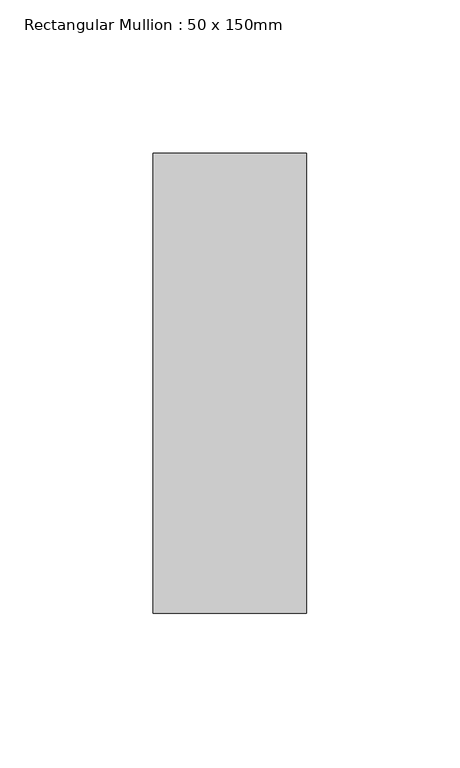
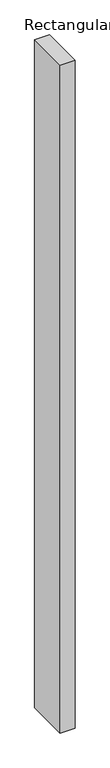
"""IFC4 building model written with IfcOpenShell, lengths in millimetres: member geometry, Rectangular Mullion : 50 x 150mm."""

from ifc_helpers import new_model, si_unit, frame, origin, place, context, project, spatial, polyline, outline, extrude, source, transform, mapped, element, save


def rectangular_mullion_50_x_150mm_662c37b1(model_context):
    return source(origin(), model_context, "Body", "SweptSolid", [
        extrude(outline(polyline([(0.0, 75.0), (0.0, -75.0), (-50.0, -75.0), (-50.0, 75.0), (0.0, 75.0)])), frame((0.0, 0.0, -2400.0), z_axis=(0.0, 0.0, 1.0), x_axis=(1.0, 0.0, 0.0)), (0.0, 0.0, 1.0), 2400.0),
    ])


if __name__ == "__main__":
    model = new_model("IFC4")
    model_context = context("Model", 3, world=origin())
    ifc_project = project(units=[si_unit("LENGTHUNIT", "METRE", prefix="MILLI")], contexts=[model_context])
    site = spatial("IfcSite", under=ifc_project)
    building = spatial("IfcBuilding", under=site)
    placement = place(None, origin())
    rectangular_mullion_50_x_150mm_shape = rectangular_mullion_50_x_150mm_662c37b1(model_context)
    element("IfcMember", 1, ObjectType="Rectangular Mullion : 50 x 150mm", at=placement, inside=building, context=model_context, shape_type="MappedRepresentation", body=[
        mapped(rectangular_mullion_50_x_150mm_shape, transform((0.0, 0.0, 0.0), x_axis=(1.0, 0.0, 0.0), y_axis=(0.0, 1.0, 0.0), z_axis=(0.0, 0.0, 1.0))),
    ])
    save(model, "model.ifc")

# Revit data of these elements
# Type "Rectangular Mullion : 50 x 150mm"
#   built-in parameter 1007304 = 0.492126 (stored number, unit not read)
#   built-in parameter 1007301 = 0.082021 (stored number, unit not read)
#   built-in parameter 1007300 = 0.082021 (stored number, unit not read)
# Element 1 (IfcMember, "Rectangular Mullion : 50 x 150mm")
#   Materials on its faces: "Aluminium"
# Materials
#   "Aluminium": class "Metal", colour RGB 247 247 247, transparency 0, Description = "Aluminium 6061", Cost = 0
